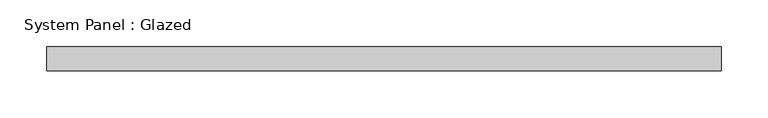
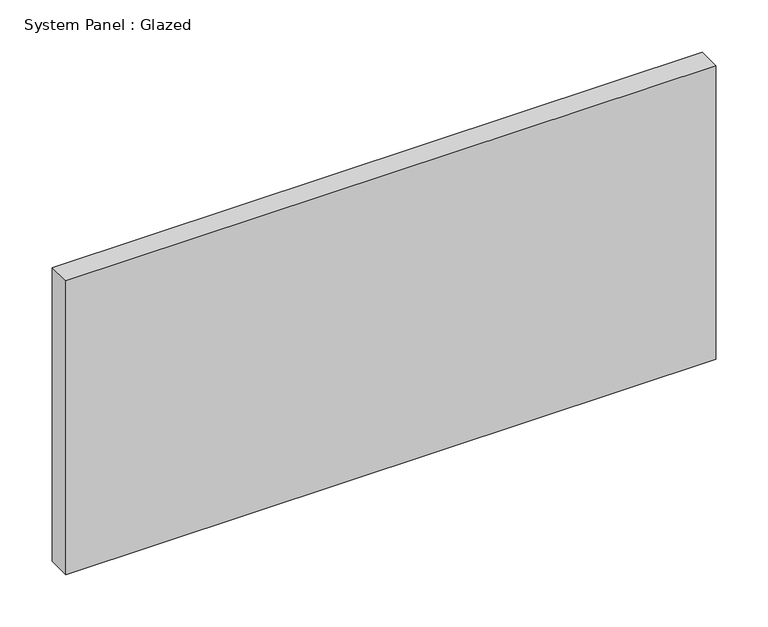
"""IFC4 building model written with IfcOpenShell, lengths in millimetres: plate geometry, System Panel : Glazed."""

from ifc_helpers import new_model, si_unit, origin, origin_with_axes, place, context, project, spatial, polyline, outline, extrude, source, transform, mapped, element, save


def system_panel_glazed_ef4f0122(model_context):
    return source(origin(), model_context, "Body", "SweptSolid", [
        extrude(outline(polyline([(358.775, 19.05), (-358.775, 19.05), (-358.775, 44.45), (358.775, 44.45), (358.775, 19.05)])), origin_with_axes(), (0.0, 0.0, 1.0), 342.9),
    ])


if __name__ == "__main__":
    model = new_model("IFC4")
    model_context = context("Model", 3, world=origin())
    ifc_project = project(units=[si_unit("LENGTHUNIT", "METRE", prefix="MILLI")], contexts=[model_context])
    site = spatial("IfcSite", under=ifc_project)
    building = spatial("IfcBuilding", under=site)
    placement = place(None, origin())
    system_panel_glazed_shape = system_panel_glazed_ef4f0122(model_context)
    element("IfcPlate", 1, ObjectType="System Panel : Glazed", at=placement, inside=building, context=model_context, shape_type="MappedRepresentation", body=[
        mapped(system_panel_glazed_shape, transform((0.0, 0.0, 0.0), x_axis=(1.0, 0.0, 0.0), y_axis=(0.0, 1.0, 0.0), z_axis=(0.0, 0.0, 1.0))),
    ])
    save(model, "model.ifc")

# Revit data of these elements
# Type "System Panel : Glazed"
#   Construction Type Id = "GSP4R"
#   Analytic Construction = "1/8 in Pilkington single glazing"
#   Visual Light Transmittance = 0.9
#   Solar Heat Gain Coefficient = 0.86
#   Heat Transfer Coefficient (U) = 1.18115 BTU/(h·ft²·°F)
#   Define Thermal Properties by = 1
# Element 1 (IfcPlate, "System Panel : Glazed")
#   Materials on its faces: "Glass"
# Materials
#   "Glass": class "Glass", colour RGB 0 128 192, transparency 0.75, Description = "Soda Lime Glass", Cost = 0
